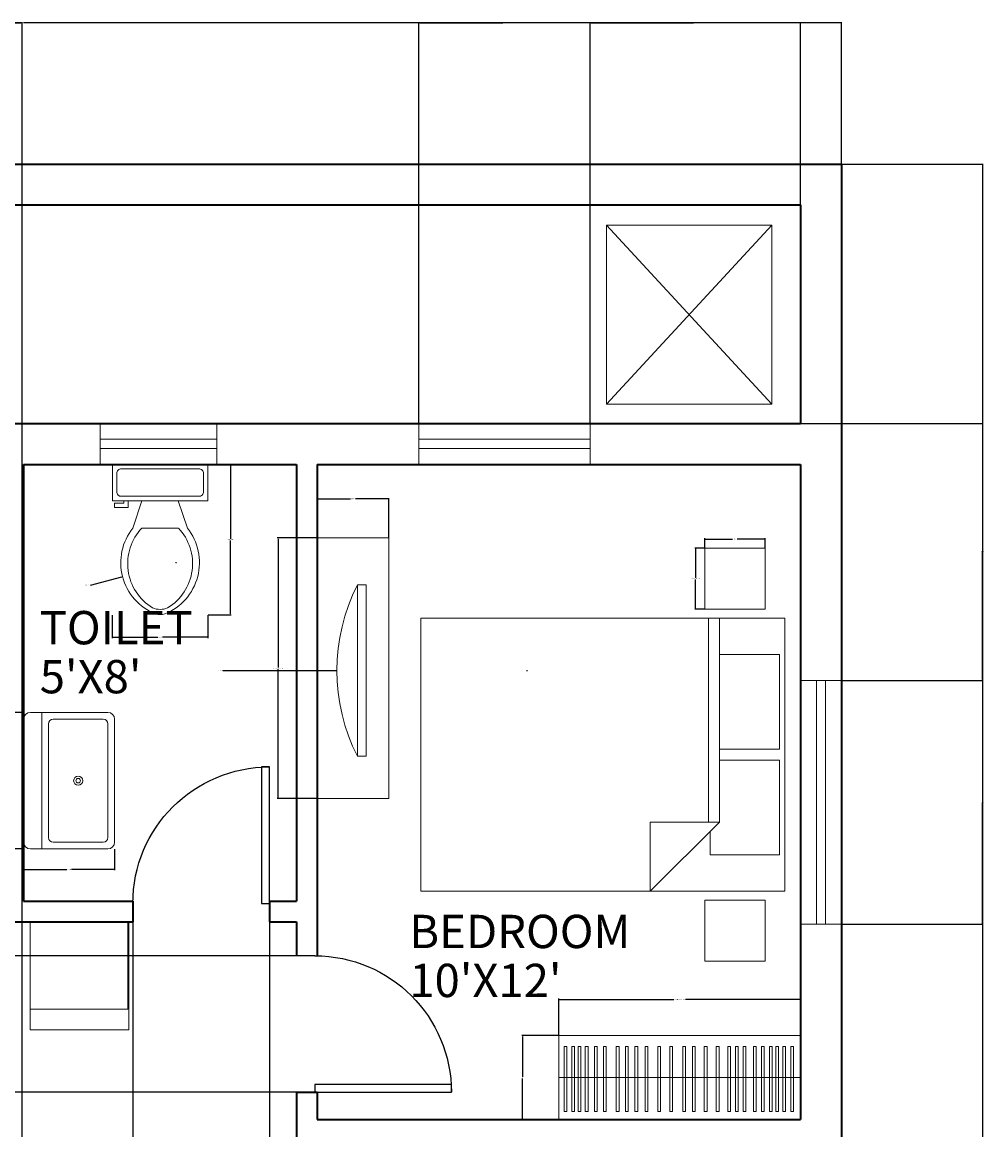
# Model space of a CAD drawing. Units: inches. Extents: x 25018 to 25490, y 41421 to 42101.
# Tile 5 of 5: x 25279 to 25490, y 41858 to 42101. Entities that reach past the tile are written whole.
import ezdxf

# ---------------------------------------------------------------- set-up
doc = ezdxf.new("R2010")
doc.units = ezdxf.units.IN
for name, color, linetype, lineweight in [('A-ANNO-DIMS', 2, 'Continuous', 18), ('A-AREA-IDEN', 7, 'Continuous', 18), ('A-DOOR', 3, 'Continuous', 25), ('A-FLOR-FIXT', 9, 'Continuous', 18), ('A-FURN', 8, 'Continuous', 18), ('A-GLAZ', 4, 'Continuous', 18), ('A-WALL', 7, 'Continuous', 35)]:
    doc.layers.add(name, color=color, linetype=linetype, lineweight=lineweight)
doc.styles.get("Standard").update_dxf_attribs({"font": 'arial.ttf'})
doc.dimstyles.get("Standard").update_dxf_attribs({"dimtxt": 0.18, "dimasz": 0.18, "dimexe": 0.18, "dimexo": 0.0625, "dimgap": 0.09, "dimtad": 0, "dimtih": 1, "dimtoh": 1, "dimdec": 4, "dimzin": 0, "dimdsep": 46, "dimtxsty": 'Standard', "dimcen": 0.09, "dimadec": 0, "dimazin": 0, "dimtfac": 1, "dimtdec": 4, "dimtofl": 0, "dimtmove": 0, "dimatfit": 3, "dimfxl": 1, "dimtolj": 1, "dimtzin": 0, "dimarcsym": 0})

# ---------------------------------------------------------------- blocks, each defined once
blk = doc.blocks.new('*U2')
for p, q in [((0, 0), (0, -100)), ((750, 0), (750, -100))]:
    blk.add_line(p, q)
blk.add_lwpolyline([(0, 0), (0, 750), (43.75, 750), (43.75, 0)], close=True)
blk.add_arc((0, 0), 750, 0, 90)
blk = doc.blocks.new('Toilet - top')
for p, q in [((9.5, -6), (9.5, -2)), ((-10, -8.5), (-8, -8.5)), ((-10, -9.5), (-10, -8.5)), ((-7, -9.5), (-10, -9.5)), ((-8, -8.5), (-8, -8)), ((-7, -8), (-7, -9.5)), ((-4, -8), (-6, -14)), ((4, -8), (6, -14)), ((4, -14), (-4, -14))]:
    blk.add_line(p, q)
blk.add_lwpolyline([(10.5, -8), (10.5, 0), (-10.5, 0), (-10.5, -8)], close=True)
for points in [[(-9.5, -2), (-9.5, -6)], [(8.5, -1), (-8.5, -1)], [(-8.5, -7), (8.5, -7)]]:
    blk.add_lwpolyline(points)
for centre, radius, start, end in [((-8.62, -1.88), 0.884, 81.8699, 188.1301), ((8.62, -1.88), 0.884, 351.8699, 98.1301), ((-8.62, -6.12), 0.884, 171.8699, 278.1301), ((8.62, -6.12), 0.884, 261.8699, 8.1301), ((3.52, -21.58), 12.17, 141.4691, 247.9714), ((4.2, -21.82), 11.33, 136.3677, 238.9468), ((-3.52, -21.58), 12.17, 292.0284, 38.5307), ((-4.2, -21.82), 11.33, 301.053, 43.6321), ((0, -27.88), 4, 245.7318, 294.2682), ((0, -29), 4, 254.8605, 285.1395)]:
    blk.add_arc(centre, radius, start, end)
blk = doc.blocks.new('Sink-single - 30 in top')
blk.add_line((-15, -3.999996), (15, -3.999996))
for points in [[(-13.5, 0), (13.5, 0)], [(-15, -18.499996), (-15, -1.5)], [(15, -1.5), (15, -18.499996)], [(-13.5, -17.499996), (-13.5, -6.499996)], [(-12.5, -5.499996), (12.5, -5.499996)], [(13.5, -6.499996), (13.5, -17.499996)], [(12.5, -18.499996), (-12.5, -18.499996)], [(13.5, -19.999996), (-13.5, -19.999996)]]:
    blk.add_lwpolyline(points)
for radius in [1, 0.5]:
    blk.add_circle((0, -11.999996), radius)
for centre, radius, start, end in [((-13.5, -1.5), 1.5, 90, 180), ((13.5, -1.5), 1.5, 0, 90), ((-12.5, -6.499996), 1, 90, 180), ((12.5, -6.499996), 1, 0, 90), ((-13.5, -18.499996), 1.5, 180, 270), ((-12.5, -17.499996), 1, 180, 270), ((12.5, -17.499996), 1, 270, 0), ((13.5, -18.499996), 1.5, 270, 0)]:
    blk.add_arc(centre, radius, start, end)
blk = doc.blocks.new('Bed - Queen')
for p, q in [((0, -80.00003), (0, 0)), ((0, 0), (59.99999, 0)), ((59.99999, 0), (59.99999, -80.00003)), ((7.99999, -1.2), (28.79998, -1.2)), ((7.99999, -14.4), (7.99999, -1.2)), ((28.79998, -1.2), (28.79998, -14.4)), ((31.19999, -1.2), (51.99999, -1.2)), ((31.19999, -14.4), (31.19999, -1.2)), ((51.99999, -1.2), (51.99999, -16.4)), ((0, -14.4), (44.8, -14.4)), ((59.99999, -29.6), (44.8, -14.4)), ((44.8, -14.4), (44.8, -29.6)), ((44.8, -16.8), (0, -16.8)), ((51.99999, -16.4), (46.79936, -16.4)), ((44.8, -29.6), (59.99999, -29.6)), ((59.99999, -80.00003), (0, -80.00003))]:
    blk.add_line(p, q)
blk = doc.blocks.new('WARDROBE-SLATTED')
blk.add_line((0, 9.22), (53.1, 9.22))
for points in [[(0, 0), (53.1, 0), (53.1, 18.45), (0, 18.45)], [(1.16, 16.06), (1.76, 16.06), (1.76, 1.75), (1.16, 1.75)], [(2.87, 16.06), (3.47, 16.06), (3.47, 1.75), (2.87, 1.75)], [(4.23, 16.06), (4.83, 16.06), (4.83, 1.75), (4.23, 1.75)], [(5.83, 16.06), (6.43, 16.06), (6.43, 1.75), (5.83, 1.75)], [(7.85, 16.06), (8.45, 16.06), (8.45, 1.75), (7.85, 1.75)], [(9.82, 16.06), (10.42, 16.06), (10.42, 1.75), (9.82, 1.75)], [(12.64, 16.06), (13.24, 16.06), (13.24, 1.75), (12.64, 1.75)], [(14.63, 16.06), (15.23, 16.06), (15.23, 1.75), (14.63, 1.75)], [(16.74, 16.06), (17.34, 16.06), (17.34, 1.75), (16.74, 1.75)], [(18.99, 16.06), (19.59, 16.06), (19.59, 1.75), (18.99, 1.75)], [(21.77, 16.06), (22.37, 16.06), (22.37, 1.75), (21.77, 1.75)], [(24.4, 16.06), (25, 16.06), (25, 1.75), (24.4, 1.75)], [(27.25, 16.06), (27.85, 16.06), (27.85, 1.75), (27.25, 1.75)], [(29.36, 16.06), (29.96, 16.06), (29.96, 1.75), (29.36, 1.75)], [(31.98, 16.06), (32.58, 16.06), (32.58, 1.75), (31.98, 1.75)], [(34.61, 16.06), (35.21, 16.06), (35.21, 1.75), (34.61, 1.75)], [(37.17, 16.06), (37.77, 16.06), (37.77, 1.75), (37.17, 1.75)], [(38.82, 16.06), (39.42, 16.06), (39.42, 1.75), (38.82, 1.75)], [(40.51, 16.06), (41.11, 16.06), (41.11, 1.75), (40.51, 1.75)], [(42.78, 16.06), (43.38, 16.06), (43.38, 1.75), (42.78, 1.75)], [(44.55, 16.06), (45.15, 16.06), (45.15, 1.75), (44.55, 1.75)], [(46.32, 16.06), (46.92, 16.06), (46.92, 1.75), (46.32, 1.75)], [(47.7, 16.06), (48.3, 16.06), (48.3, 1.75), (47.7, 1.75)], [(49.2, 16.06), (49.8, 16.06), (49.8, 1.75), (49.2, 1.75)], [(50.97, 16.06), (51.57, 16.06), (51.57, 1.75), (50.97, 1.75)]]:
    blk.add_lwpolyline(points, close=True)
blk = doc.blocks.new('TABLE-BEDSIDE')
blk.add_lwpolyline([(0, 13.4), (13.26, 13.4), (13.26, 0), (0, 0)], close=True)
blk = doc.blocks.new('TV-CONSOLE')
for points in [[(0, 57.27), (15.78, 57.27), (15.78, 0), (0, 0)], [(8.85, 46.95), (10.77, 46.95), (10.77, 9.28), (8.85, 9.28)]]:
    blk.add_lwpolyline(points, close=True)
blk.add_arc((46.16, 28.12), 41.8, 153.2115, 206.7885)
blk = doc.blocks.new('WIN-BATH')
for p, q in [((0, 9), (0, 0)), ((25.67, 0), (25.67, 9)), ((0, 5.5), (25.67, 5.5)), ((0, 3.5), (25.67, 3.5))]:
    blk.add_line(p, q)
blk = doc.blocks.new('*D20')
at = {"layer": 'A-ANNO-DIMS', "color": 0, "lineweight": -2, "transparency": 16777216}
for p, q in [((25396.55, 41878.56), (25396.55, 41886.64)), ((25396.73, 41886.46), (25421.8, 41886.46)), ((25449.47, 41886.46), (25424.41, 41886.46)), ((25449.65, 41878.56), (25449.65, 41886.64))]:
    blk.add_line(p, q, dxfattribs=at)
at = {"layer": 'A-ANNO-DIMS', "color": 0, "transparency": 16777216}
for points in [[(25396.73, 41886.49), (25396.73, 41886.43), (25396.55, 41886.46)], [(25449.47, 41886.49), (25449.47, 41886.43), (25449.65, 41886.46)]]:
    blk.add_solid(points, dxfattribs=at)
at = {"layer": 'Defpoints', "color": 0, "transparency": 16777216}
for p in [(25449.65, 41886.46), (25396.55, 41878.5), (25449.65, 41878.5)]:
    blk.add_point(p, dxfattribs=at)
at = {"layer": 'A-ANNO-DIMS', "color": 0, "transparency": 16777216, "insert": (25423.1, 41886.46), "char_height": 0.18, "attachment_point": 5}
blk.add_mtext('\\A1;WARDROBE 53 TYP.', dxfattribs=at)
blk = doc.blocks.new('*D21')
at = {"layer": 'A-ANNO-DIMS', "color": 0, "lineweight": -2, "transparency": 16777216}
for p, q in [((25396.49, 41878.5), (25388.41, 41878.5)), ((25388.59, 41878.32), (25388.59, 41869.46)), ((25388.59, 41860.23), (25388.59, 41869.09)), ((25396.49, 41860.05), (25388.41, 41860.05))]:
    blk.add_line(p, q, dxfattribs=at)
at = {"layer": 'A-ANNO-DIMS', "color": 0, "transparency": 16777216}
for points in [[(25388.56, 41878.32), (25388.62, 41878.32), (25388.59, 41878.5)], [(25388.56, 41860.23), (25388.62, 41860.23), (25388.59, 41860.05)]]:
    blk.add_solid(points, dxfattribs=at)
at = {"layer": 'Defpoints', "color": 0, "transparency": 16777216}
for p in [(25388.59, 41878.5), (25396.55, 41878.5), (25396.55, 41860.05)]:
    blk.add_point(p, dxfattribs=at)
at = {"layer": 'A-ANNO-DIMS', "color": 0, "transparency": 16777216, "insert": (25388.59, 41869.27), "char_height": 0.18, "attachment_point": 5}
blk.add_mtext('\\A1;18 TYP.', dxfattribs=at)
blk = doc.blocks.new('*D22')
at = {"layer": 'A-ANNO-DIMS', "color": 0, "lineweight": -2, "transparency": 16777216}
for p, q in [((25428.57, 41985.63), (25426.44, 41985.63)), ((25426.62, 41985.45), (25426.62, 41979.12)), ((25426.62, 41972.41), (25426.62, 41978.75)), ((25428.57, 41972.23), (25426.44, 41972.23))]:
    blk.add_line(p, q, dxfattribs=at)
at = {"layer": 'A-ANNO-DIMS', "color": 0, "transparency": 16777216}
for points in [[(25426.59, 41985.45), (25426.65, 41985.45), (25426.62, 41985.63)], [(25426.59, 41972.41), (25426.65, 41972.41), (25426.62, 41972.23)]]:
    blk.add_solid(points, dxfattribs=at)
at = {"layer": 'Defpoints', "color": 0, "transparency": 16777216}
for p in [(25426.62, 41985.63), (25428.63, 41985.63), (25428.63, 41972.23)]:
    blk.add_point(p, dxfattribs=at)
at = {"layer": 'A-ANNO-DIMS', "color": 0, "transparency": 16777216, "insert": (25426.62, 41978.93), "char_height": 0.18, "attachment_point": 5}
blk.add_mtext('\\A1;NIGHTSTAND 13 TYP.', dxfattribs=at)
blk = doc.blocks.new('*D23')
at = {"layer": 'A-ANNO-DIMS', "color": 0, "lineweight": -2, "transparency": 16777216}
for p, q in [((25428.63, 41985.7), (25428.63, 41987.82)), ((25428.81, 41987.64), (25434.74, 41987.64)), ((25441.71, 41987.64), (25435.78, 41987.64)), ((25441.89, 41985.7), (25441.89, 41987.82))]:
    blk.add_line(p, q, dxfattribs=at)
at = {"layer": 'A-ANNO-DIMS', "color": 0, "transparency": 16777216}
for points in [[(25428.81, 41987.67), (25428.81, 41987.61), (25428.63, 41987.64)], [(25441.71, 41987.67), (25441.71, 41987.61), (25441.89, 41987.64)]]:
    blk.add_solid(points, dxfattribs=at)
at = {"layer": 'Defpoints', "color": 0, "transparency": 16777216}
for p in [(25441.89, 41987.64), (25428.63, 41985.63), (25441.89, 41985.63)]:
    blk.add_point(p, dxfattribs=at)
at = {"layer": 'A-ANNO-DIMS', "color": 0, "transparency": 16777216, "insert": (25435.26, 41987.64), "char_height": 0.18, "attachment_point": 5}
blk.add_mtext('\\A1;13 TYP.', dxfattribs=at)
blk = doc.blocks.new('*D24')
at = {"layer": 'A-ANNO-DIMS', "color": 0, "lineweight": -2, "transparency": 16777216}
for p, q in [((25343.39, 41987.88), (25334.68, 41987.88)), ((25334.86, 41987.7), (25334.86, 41959.43)), ((25334.86, 41930.79), (25334.86, 41959.06)), ((25343.39, 41930.61), (25334.68, 41930.61))]:
    blk.add_line(p, q, dxfattribs=at)
at = {"layer": 'A-ANNO-DIMS', "color": 0, "transparency": 16777216}
for points in [[(25334.83, 41987.7), (25334.89, 41987.7), (25334.86, 41987.88)], [(25334.83, 41930.79), (25334.89, 41930.79), (25334.86, 41930.61)]]:
    blk.add_solid(points, dxfattribs=at)
at = {"layer": 'Defpoints', "color": 0, "transparency": 16777216}
for p in [(25334.86, 41987.88), (25343.45, 41987.88), (25343.45, 41930.61)]:
    blk.add_point(p, dxfattribs=at)
at = {"layer": 'A-ANNO-DIMS', "color": 0, "transparency": 16777216, "insert": (25334.86, 41959.24), "char_height": 0.18, "attachment_point": 5}
blk.add_mtext('\\A1;TV CONSOLE 57 TYP.', dxfattribs=at)
blk = doc.blocks.new('*D25')
at = {"layer": 'A-ANNO-DIMS', "color": 0, "lineweight": -2, "transparency": 16777216}
for p, q in [((25343.45, 41987.94), (25343.45, 41996.65)), ((25359.23, 41987.94), (25359.23, 41996.65)), ((25343.63, 41996.47), (25350.82, 41996.47)), ((25359.05, 41996.47), (25351.86, 41996.47))]:
    blk.add_line(p, q, dxfattribs=at)
at = {"layer": 'A-ANNO-DIMS', "color": 0, "transparency": 16777216}
for points in [[(25343.63, 41996.5), (25343.63, 41996.44), (25343.45, 41996.47)], [(25359.05, 41996.5), (25359.05, 41996.44), (25359.23, 41996.47)]]:
    blk.add_solid(points, dxfattribs=at)
at = {"layer": 'Defpoints', "color": 0, "transparency": 16777216}
for p in [(25359.23, 41996.47), (25343.45, 41987.88), (25359.23, 41987.88)]:
    blk.add_point(p, dxfattribs=at)
at = {"layer": 'A-ANNO-DIMS', "color": 0, "transparency": 16777216, "insert": (25351.34, 41996.47), "char_height": 0.18, "attachment_point": 5}
blk.add_mtext('\\A1;16 TYP.', dxfattribs=at)
blk = doc.blocks.new('*D28')
at = {"layer": 'A-ANNO-DIMS', "color": 0, "lineweight": -2, "transparency": 16777216}
for p, q in [((25319.52, 42004.05), (25324.59, 42004.05)), ((25324.41, 42003.87), (25324.41, 41987.71)), ((25324.41, 41971.18), (25324.41, 41987.34)), ((25319.52, 41971), (25324.59, 41971))]:
    blk.add_line(p, q, dxfattribs=at)
at = {"layer": 'A-ANNO-DIMS', "color": 0, "transparency": 16777216}
for points in [[(25324.38, 42003.87), (25324.44, 42003.87), (25324.41, 42004.05)], [(25324.38, 41971.18), (25324.44, 41971.18), (25324.41, 41971)]]:
    blk.add_solid(points, dxfattribs=at)
at = {"layer": 'Defpoints', "color": 0, "transparency": 16777216}
for p in [(25319.45, 42004.05), (25324.41, 42004.05), (25319.45, 41971)]:
    blk.add_point(p, dxfattribs=at)
at = {"layer": 'A-ANNO-DIMS', "color": 0, "transparency": 16777216, "insert": (25324.41, 41987.53), "char_height": 0.18, "attachment_point": 5}
blk.add_mtext('\\A1;WC 33 TYP.', dxfattribs=at)
blk = doc.blocks.new('*D29')
at = {"layer": 'A-ANNO-DIMS', "color": 0, "lineweight": -2, "transparency": 16777216}
for p, q in [((25298.45, 41970.94), (25298.45, 41965.87)), ((25319.45, 41970.94), (25319.45, 41965.87)), ((25298.63, 41966.05), (25308.42, 41966.05)), ((25319.27, 41966.05), (25309.48, 41966.05))]:
    blk.add_line(p, q, dxfattribs=at)
at = {"layer": 'A-ANNO-DIMS', "color": 0, "transparency": 16777216}
for points in [[(25298.63, 41966.08), (25298.63, 41966.02), (25298.45, 41966.05)], [(25319.27, 41966.08), (25319.27, 41966.02), (25319.45, 41966.05)]]:
    blk.add_solid(points, dxfattribs=at)
at = {"layer": 'Defpoints', "color": 0, "transparency": 16777216}
for p in [(25298.45, 41971), (25319.45, 41971), (25319.45, 41966.05)]:
    blk.add_point(p, dxfattribs=at)
at = {"layer": 'A-ANNO-DIMS', "color": 0, "transparency": 16777216, "insert": (25308.95, 41966.05), "char_height": 0.18, "attachment_point": 5}
blk.add_mtext('\\A1;21 TYP.', dxfattribs=at)
blk = doc.blocks.new('*D30')
at = {"layer": 'A-ANNO-DIMS', "color": 0, "lineweight": -2, "transparency": 16777216}
for p, q in [((25278.89, 41949.53), (25274.27, 41949.53)), ((25274.45, 41949.35), (25274.45, 41934.71)), ((25274.45, 41919.71), (25274.45, 41934.35)), ((25278.89, 41919.53), (25274.27, 41919.53))]:
    blk.add_line(p, q, dxfattribs=at)
at = {"layer": 'A-ANNO-DIMS', "color": 0, "transparency": 16777216}
for points in [[(25274.42, 41949.35), (25274.48, 41949.35), (25274.45, 41949.53)], [(25274.42, 41919.71), (25274.48, 41919.71), (25274.45, 41919.53)]]:
    blk.add_solid(points, dxfattribs=at)
at = {"layer": 'Defpoints', "color": 0, "transparency": 16777216}
for p in [(25274.45, 41949.53), (25278.95, 41949.53), (25278.95, 41919.53)]:
    blk.add_point(p, dxfattribs=at)
at = {"layer": 'A-ANNO-DIMS', "color": 0, "transparency": 16777216, "insert": (25274.45, 41934.53), "char_height": 0.18, "attachment_point": 5}
blk.add_mtext('\\A1;BASIN 30 TYP.', dxfattribs=at)
blk = doc.blocks.new('*D31')
at = {"layer": 'A-ANNO-DIMS', "color": 0, "lineweight": -2, "transparency": 16777216}
for p, q in [((25278.95, 41919.47), (25278.95, 41914.85)), ((25298.95, 41919.47), (25298.95, 41914.85)), ((25279.13, 41915.03), (25288.42, 41915.03)), ((25298.77, 41915.03), (25289.48, 41915.03))]:
    blk.add_line(p, q, dxfattribs=at)
at = {"layer": 'A-ANNO-DIMS', "color": 0, "transparency": 16777216}
for points in [[(25279.13, 41915.06), (25279.13, 41915), (25278.95, 41915.03)], [(25298.77, 41915.06), (25298.77, 41915), (25298.95, 41915.03)]]:
    blk.add_solid(points, dxfattribs=at)
at = {"layer": 'Defpoints', "color": 0, "transparency": 16777216}
for p in [(25278.95, 41919.53), (25298.95, 41919.53), (25278.95, 41915.03)]:
    blk.add_point(p, dxfattribs=at)
at = {"layer": 'A-ANNO-DIMS', "color": 0, "transparency": 16777216, "insert": (25288.95, 41915.03), "char_height": 0.18, "attachment_point": 5}
blk.add_mtext('\\A1;20 TYP.', dxfattribs=at)
blk = doc.blocks.new('*D38')
at = {"layer": 'A-ANNO-DIMS', "color": 0, "lineweight": -2, "transparency": 16777216}
for p, q in [((25098.65, 42070.11), (25098.65, 42101.23)), ((25458.65, 42070.11), (25458.65, 42101.23)), ((25098.83, 42101.05), (25278.36, 42101.05)), ((25458.47, 42101.05), (25278.94, 42101.05))]:
    blk.add_line(p, q, dxfattribs=at)
at = {"layer": 'A-ANNO-DIMS', "color": 0, "transparency": 16777216}
for points in [[(25098.83, 42101.08), (25098.83, 42101.02), (25098.65, 42101.05)], [(25458.47, 42101.08), (25458.47, 42101.02), (25458.65, 42101.05)]]:
    blk.add_solid(points, dxfattribs=at)
at = {"layer": 'Defpoints', "color": 0, "transparency": 16777216}
for p in [(25458.65, 42101.05), (25098.65, 42070.05), (25458.65, 42070.05)]:
    blk.add_point(p, dxfattribs=at)
at = {"layer": 'A-ANNO-DIMS', "color": 0, "transparency": 16777216, "insert": (25278.65, 42101.05), "char_height": 0.18, "attachment_point": 5}
blk.add_mtext('\\A1;360', dxfattribs=at)
blk = doc.blocks.new('*D39')
at = {"layer": 'A-ANNO-DIMS', "color": 0, "lineweight": -2, "transparency": 16777216}
for p, q in [((25458.72, 42070.05), (25489.83, 42070.05)), ((25489.65, 42069.87), (25489.65, 41785.98)), ((25489.65, 41501.73), (25489.65, 41785.62)), ((25458.72, 41501.55), (25489.83, 41501.55))]:
    blk.add_line(p, q, dxfattribs=at)
at = {"layer": 'A-ANNO-DIMS', "color": 0, "transparency": 16777216}
for points in [[(25489.62, 42069.87), (25489.68, 42069.87), (25489.65, 42070.05)], [(25489.62, 41501.73), (25489.68, 41501.73), (25489.65, 41501.55)]]:
    blk.add_solid(points, dxfattribs=at)
at = {"layer": 'Defpoints', "color": 0, "transparency": 16777216}
for p in [(25458.65, 42070.05), (25489.65, 42070.05), (25458.65, 41501.55)]:
    blk.add_point(p, dxfattribs=at)
at = {"layer": 'A-ANNO-DIMS', "color": 0, "transparency": 16777216, "insert": (25489.65, 41785.8), "char_height": 0.18, "attachment_point": 5}
blk.add_mtext('\\A1;568.5', dxfattribs=at)
blk = doc.blocks.new('*D56')
at = {"layer": 'A-ANNO-DIMS', "color": 0, "lineweight": -2, "transparency": 16777216}
for p, q in [((25458.72, 41903), (25489.83, 41903)), ((25489.65, 41902.82), (25489.65, 41855.5)), ((25489.65, 41807.81), (25489.65, 41855.13)), ((25458.72, 41807.63), (25489.83, 41807.63))]:
    blk.add_line(p, q, dxfattribs=at)
at = {"layer": 'A-ANNO-DIMS', "color": 0, "transparency": 16777216}
for points in [[(25489.62, 41902.82), (25489.68, 41902.82), (25489.65, 41903)], [(25489.62, 41807.81), (25489.68, 41807.81), (25489.65, 41807.63)]]:
    blk.add_solid(points, dxfattribs=at)
at = {"layer": 'Defpoints', "color": 0, "transparency": 16777216}
for p in [(25458.65, 41903), (25489.65, 41903), (25458.65, 41807.63)]:
    blk.add_point(p, dxfattribs=at)
at = {"layer": 'A-ANNO-DIMS', "color": 0, "transparency": 16777216, "insert": (25489.65, 41855.31), "char_height": 0.18, "attachment_point": 5}
blk.add_mtext('\\A1;95.36', dxfattribs=at)
blk = doc.blocks.new('*D57')
at = {"layer": 'A-ANNO-DIMS', "color": 0, "lineweight": -2, "transparency": 16777216}
for p, q in [((25458.72, 41956.57), (25489.83, 41956.57)), ((25489.65, 41956.39), (25489.65, 41929.96)), ((25489.65, 41903.18), (25489.65, 41929.6)), ((25458.72, 41903), (25489.83, 41903))]:
    blk.add_line(p, q, dxfattribs=at)
at = {"layer": 'A-ANNO-DIMS', "color": 0, "transparency": 16777216}
for points in [[(25489.62, 41956.39), (25489.68, 41956.39), (25489.65, 41956.57)], [(25489.62, 41903.18), (25489.68, 41903.18), (25489.65, 41903)]]:
    blk.add_solid(points, dxfattribs=at)
at = {"layer": 'Defpoints', "color": 0, "transparency": 16777216}
for p in [(25458.65, 41956.57), (25489.65, 41956.57), (25458.65, 41903)]:
    blk.add_point(p, dxfattribs=at)
at = {"layer": 'A-ANNO-DIMS', "color": 0, "transparency": 16777216, "insert": (25489.65, 41929.78), "char_height": 0.18, "attachment_point": 5}
blk.add_mtext('\\A1;53.57', dxfattribs=at)
blk = doc.blocks.new('*D58')
at = {"layer": 'A-ANNO-DIMS', "color": 0, "lineweight": -2, "transparency": 16777216}
for p, q in [((25449.72, 42013.05), (25489.83, 42013.05)), ((25489.65, 42012.87), (25489.65, 41984.99)), ((25489.65, 41956.75), (25489.65, 41984.63)), ((25458.72, 41956.57), (25489.83, 41956.57))]:
    blk.add_line(p, q, dxfattribs=at)
at = {"layer": 'A-ANNO-DIMS', "color": 0, "transparency": 16777216}
for points in [[(25489.62, 42012.87), (25489.68, 42012.87), (25489.65, 42013.05)], [(25489.62, 41956.75), (25489.68, 41956.75), (25489.65, 41956.57)]]:
    blk.add_solid(points, dxfattribs=at)
at = {"layer": 'Defpoints', "color": 0, "transparency": 16777216}
for p in [(25449.65, 42013.05), (25489.65, 42013.05), (25458.65, 41956.57)]:
    blk.add_point(p, dxfattribs=at)
at = {"layer": 'A-ANNO-DIMS', "color": 0, "transparency": 16777216, "insert": (25489.65, 41984.81), "char_height": 0.18, "attachment_point": 5}
blk.add_mtext('\\A1;56.48', dxfattribs=at)
blk = doc.blocks.new('*D64')
at = {"layer": 'A-ANNO-DIMS', "color": 0, "lineweight": -2, "transparency": 16777216}
for p, q in [((25365.82, 42013.11), (25365.82, 42101.23)), ((25403.48, 42013.11), (25403.48, 42101.23)), ((25366, 42101.05), (25384.26, 42101.05)), ((25403.3, 42101.05), (25385.05, 42101.05))]:
    blk.add_line(p, q, dxfattribs=at)
at = {"layer": 'A-ANNO-DIMS', "color": 0, "transparency": 16777216}
for points in [[(25366, 42101.08), (25366, 42101.02), (25365.82, 42101.05)], [(25403.3, 42101.08), (25403.3, 42101.02), (25403.48, 42101.05)]]:
    blk.add_solid(points, dxfattribs=at)
at = {"layer": 'Defpoints', "color": 0, "transparency": 16777216}
for p in [(25403.48, 42101.05), (25365.82, 42013.05), (25403.48, 42013.05)]:
    blk.add_point(p, dxfattribs=at)
at = {"layer": 'A-ANNO-DIMS', "color": 0, "transparency": 16777216, "insert": (25384.65, 42101.05), "char_height": 0.18, "attachment_point": 5}
blk.add_mtext('\\A1;37.66', dxfattribs=at)
blk = doc.blocks.new('*D65')
at = {"layer": 'A-ANNO-DIMS', "color": 0, "lineweight": -2, "transparency": 16777216}
for p, q in [((25403.48, 42013.11), (25403.48, 42101.23)), ((25449.65, 42013.11), (25449.65, 42101.23)), ((25403.66, 42101.05), (25426.17, 42101.05)), ((25449.47, 42101.05), (25426.97, 42101.05))]:
    blk.add_line(p, q, dxfattribs=at)
at = {"layer": 'A-ANNO-DIMS', "color": 0, "transparency": 16777216}
for points in [[(25403.66, 42101.08), (25403.66, 42101.02), (25403.48, 42101.05)], [(25449.47, 42101.08), (25449.47, 42101.02), (25449.65, 42101.05)]]:
    blk.add_solid(points, dxfattribs=at)
at = {"layer": 'Defpoints', "color": 0, "transparency": 16777216}
for p in [(25449.65, 42101.05), (25403.48, 42013.05), (25449.65, 42013.05)]:
    blk.add_point(p, dxfattribs=at)
at = {"layer": 'A-ANNO-DIMS', "color": 0, "transparency": 16777216, "insert": (25426.57, 42101.05), "char_height": 0.18, "attachment_point": 5}
blk.add_mtext('\\A1;46.17', dxfattribs=at)
blk = doc.blocks.new('*D70')
at = {"layer": 'A-ANNO-DIMS', "color": 0, "lineweight": -2, "transparency": 16777216}
for p, q in [((25250.45, 41903.49), (25250.45, 41420.7)), ((25302.95, 41903.49), (25302.95, 41420.7)), ((25250.63, 41420.88), (25276.38, 41420.88)), ((25302.77, 41420.88), (25277.03, 41420.88))]:
    blk.add_line(p, q, dxfattribs=at)
at = {"layer": 'A-ANNO-DIMS', "color": 0, "transparency": 16777216}
for points in [[(25250.63, 41420.91), (25250.63, 41420.85), (25250.45, 41420.88)], [(25302.77, 41420.91), (25302.77, 41420.85), (25302.95, 41420.88)]]:
    blk.add_solid(points, dxfattribs=at)
at = {"layer": 'Defpoints', "color": 0, "transparency": 16777216}
for p in [(25250.45, 41903.55), (25302.95, 41903.55), (25302.95, 41420.88)]:
    blk.add_point(p, dxfattribs=at)
at = {"layer": 'A-ANNO-DIMS', "color": 0, "transparency": 16777216, "insert": (25276.7, 41420.88), "char_height": 0.18, "attachment_point": 5}
blk.add_mtext('\\A1;52.5', dxfattribs=at)
blk = doc.blocks.new('*D71')
at = {"layer": 'A-ANNO-DIMS', "color": 0, "lineweight": -2, "transparency": 16777216}
for p, q in [((25302.95, 41903.49), (25302.95, 41420.7)), ((25332.95, 41903.49), (25332.95, 41420.7)), ((25303.13, 41420.88), (25317.73, 41420.88)), ((25332.77, 41420.88), (25318.17, 41420.88))]:
    blk.add_line(p, q, dxfattribs=at)
at = {"layer": 'A-ANNO-DIMS', "color": 0, "transparency": 16777216}
for points in [[(25303.13, 41420.91), (25303.13, 41420.85), (25302.95, 41420.88)], [(25332.77, 41420.91), (25332.77, 41420.85), (25332.95, 41420.88)]]:
    blk.add_solid(points, dxfattribs=at)
at = {"layer": 'Defpoints', "color": 0, "transparency": 16777216}
for p in [(25302.95, 41903.55), (25332.95, 41903.55), (25332.95, 41420.88)]:
    blk.add_point(p, dxfattribs=at)
at = {"layer": 'A-ANNO-DIMS', "color": 0, "transparency": 16777216, "insert": (25317.95, 41420.88), "char_height": 0.18, "attachment_point": 5}
blk.add_mtext('\\A1;30', dxfattribs=at)
blk = doc.blocks.new('*D72')
at = {"layer": 'A-ANNO-DIMS', "color": 0, "lineweight": -2, "transparency": 16777216}
for p, q in [((25338.89, 41896.05), (25018.58, 41896.05)), ((25018.76, 41895.87), (25018.76, 41881.23)), ((25018.76, 41866.23), (25018.76, 41880.87)), ((25338.89, 41866.05), (25018.58, 41866.05))]:
    blk.add_line(p, q, dxfattribs=at)
at = {"layer": 'A-ANNO-DIMS', "color": 0, "transparency": 16777216}
for points in [[(25018.73, 41895.87), (25018.79, 41895.87), (25018.76, 41896.05)], [(25018.73, 41866.23), (25018.79, 41866.23), (25018.76, 41866.05)]]:
    blk.add_solid(points, dxfattribs=at)
at = {"layer": 'Defpoints', "color": 0, "transparency": 16777216}
for p in [(25018.76, 41896.05), (25338.95, 41896.05), (25338.95, 41866.05)]:
    blk.add_point(p, dxfattribs=at)
at = {"layer": 'A-ANNO-DIMS', "color": 0, "transparency": 16777216, "insert": (25018.76, 41881.05), "char_height": 0.18, "attachment_point": 5}
blk.add_mtext('\\A1;30', dxfattribs=at)
blk = doc.blocks.new('*D75')
at = {"layer": 'A-ANNO-DIMS', "color": 0, "lineweight": -2, "transparency": 16777216}
for p, q in [((25201.64, 41804.94), (25201.64, 42101.23)), ((25278.63, 41804.94), (25278.63, 42101.23)), ((25201.82, 42101.05), (25239.92, 42101.05)), ((25278.45, 42101.05), (25240.36, 42101.05))]:
    blk.add_line(p, q, dxfattribs=at)
at = {"layer": 'A-ANNO-DIMS', "color": 0, "transparency": 16777216}
for points in [[(25201.82, 42101.08), (25201.82, 42101.02), (25201.64, 42101.05)], [(25278.45, 42101.08), (25278.45, 42101.02), (25278.63, 42101.05)]]:
    blk.add_solid(points, dxfattribs=at)
at = {"layer": 'Defpoints', "color": 0, "transparency": 16777216}
for p in [(25278.63, 42101.05), (25201.64, 41804.88), (25278.63, 41804.88)]:
    blk.add_point(p, dxfattribs=at)
at = {"layer": 'A-ANNO-DIMS', "color": 0, "transparency": 16777216, "insert": (25240.14, 42101.05), "char_height": 0.18, "attachment_point": 5}
blk.add_mtext('\\A1;77', dxfattribs=at)
blk = doc.blocks.new('*D77')
at = {"layer": 'A-ANNO-DIMS', "color": 0, "lineweight": -2, "transparency": 16777216}
for p, q in [((25322.74, 41958.72), (25347.64, 41958.72)), ((25389.52, 41958.72), (25389.7, 41958.72)), ((25389.61, 41958.63), (25389.61, 41958.81))]:
    blk.add_line(p, q, dxfattribs=at)
at = {"layer": 'A-ANNO-DIMS', "color": 0, "transparency": 16777216}
blk.add_solid([(25347.64, 41958.75), (25347.64, 41958.69), (25347.82, 41958.72)], dxfattribs=at)
at = {"layer": 'Defpoints', "color": 0, "transparency": 16777216}
for p in [(25347.82, 41958.72), (25389.61, 41958.72)]:
    blk.add_point(p, dxfattribs=at)
at = {"layer": 'A-ANNO-DIMS', "color": 0, "transparency": 16777216, "insert": (25322.13, 41958.72), "char_height": 0.18, "attachment_point": 5}
blk.add_mtext('\\A1;2X R41.8', dxfattribs=at)
blk = doc.blocks.new('*D78')
at = {"layer": 'A-ANNO-DIMS', "color": 0, "lineweight": -2, "transparency": 16777216}
for p, q in [((25312.38, 41982.47), (25312.56, 41982.47)), ((25312.47, 41982.38), (25312.47, 41982.56)), ((25293.64, 41977.52), (25300.53, 41979.33))]:
    blk.add_line(p, q, dxfattribs=at)
at = {"layer": 'A-ANNO-DIMS', "color": 0, "transparency": 16777216}
blk.add_solid([(25300.52, 41979.36), (25300.54, 41979.3), (25300.7, 41979.38)], dxfattribs=at)
at = {"layer": 'Defpoints', "color": 0, "transparency": 16777216}
for p in [(25312.47, 41982.47), (25300.7, 41979.38)]:
    blk.add_point(p, dxfattribs=at)
at = {"layer": 'A-ANNO-DIMS', "color": 0, "transparency": 16777216, "insert": (25292.96, 41977.52), "char_height": 0.18, "attachment_point": 5}
blk.add_mtext('\\A1;4X R12.17', dxfattribs=at)

msp = doc.modelspace()

# ---------------------------------------------------------------- linework, layer by layer
at = {"layer": 'A-FLOR-FIXT'}
for p, q in [((25407.0062, 42017.306), (25443.3638, 42056.6421)), ((25407.0062, 42056.6421), (25443.3638, 42017.306))]:
    msp.add_line(p, q, dxfattribs=at)
for points in [[(25407.0062, 42056.6421), (25443.3638, 42056.6421), (25443.3638, 42017.306), (25407.0062, 42017.306)], [(25280.4079, 41903.5498), (25301.8795, 41903.5498), (25301.8795, 41884.3127), (25280.4079, 41884.3127)], [(25280.4079, 41903.5498), (25302.0898, 41903.5498), (25302.0898, 41879.7836), (25280.4079, 41879.7836)]]:
    msp.add_lwpolyline(points, close=True, dxfattribs=at)
at = {"layer": 'A-GLAZ'}
for p, q in [((25365.8241, 42004.0498), (25365.8241, 42013.0498)), ((25403.483, 42004.0498), (25403.483, 42013.0498)), ((25365.8241, 42009.5498), (25403.483, 42009.5498)), ((25365.8241, 42007.5498), (25403.483, 42007.5498)), ((25449.6526, 41956.5665), (25458.6526, 41956.5665)), ((25453.1526, 41956.5665), (25453.1526, 41902.9968)), ((25455.1526, 41956.5665), (25455.1526, 41902.9968)), ((25449.6526, 41902.9968), (25458.6526, 41902.9968))]:
    msp.add_line(p, q, dxfattribs=at)
at = {"layer": 'A-WALL'}
for p, q in [((25098.6526, 42070.0498), (25458.6526, 42070.0498)), ((25458.6526, 42070.0498), (25458.6526, 41501.5498)), ((25107.6526, 42061.0498), (25449.6526, 42061.0498)), ((25449.6526, 42061.0498), (25449.6526, 42013.0498)), ((25115.4026, 42013.0498), (25449.6526, 42013.0498)), ((25278.9527, 42004.0498), (25278.9527, 41908.0498)), ((25278.9527, 42004.0498), (25338.9527, 42004.0498)), ((25338.9527, 42004.0498), (25338.9527, 41908.0498)), ((25343.4527, 42004.0498), (25343.4527, 41896.0457)), ((25343.4527, 42004.0498), (25449.6526, 42004.0498)), ((25449.6526, 42004.0498), (25449.6526, 41860.0498)), ((25278.9527, 41908.0498), (25302.9527, 41908.0498)), ((25302.9527, 41908.0498), (25302.9527, 41903.5498)), ((25332.9527, 41908.0498), (25332.9527, 41903.5498)), ((25332.9527, 41908.0498), (25338.9527, 41908.0498)), ((25250.4527, 41903.5498), (25302.9527, 41903.5498)), ((25332.9527, 41903.5498), (25338.9527, 41903.5498)), ((25338.9527, 41903.5498), (25338.9527, 41896.0498)), ((25338.9527, 41866.0498), (25343.4527, 41866.0498)), ((25338.9527, 41866.0498), (25338.9527, 41860.0498)), ((25343.4527, 41866.0498), (25343.4527, 41860.0498)), ((25338.9527, 41860.0498), (25338.9527, 41855.5498)), ((25343.4527, 41860.0498), (25449.6526, 41860.0498))]:
    msp.add_line(p, q, dxfattribs=at)

# ---------------------------------------------------------------- block references
at = {"layer": 'A-DOOR', "xscale": -0.0400000000000011, "yscale": 0.0400000000000011, "zscale": 0.0400000000000011}
msp.add_blockref('*U2', (25332.9527, 41907.5498), dxfattribs=at)
at = {"layer": 'A-DOOR', "xscale": -0.0400000000000011, "yscale": 0.0400000000000011, "zscale": 0.0400000000000011, "rotation": 270}
msp.add_blockref('*U2', (25342.9527, 41866.0498), dxfattribs=at)
at = {"layer": 'A-FLOR-FIXT'}
msp.add_blockref('Toilet - top', (25308.9527, 42004.0498), dxfattribs=at)
at = {"layer": 'A-FLOR-FIXT', "rotation": 90}
msp.add_blockref('Sink-single - 30 in top', (25278.9527, 41934.5291), dxfattribs=at)
at = {"layer": 'A-FURN'}
for name, p in [('TV-CONSOLE', (25343.4531, 41930.6073)), ('TABLE-BEDSIDE', (25428.629, 41972.231)), ('WARDROBE-SLATTED', (25396.553, 41860.05))]:
    msp.add_blockref(name, p, dxfattribs=at)
at = {"layer": 'A-FURN', "rotation": 270}
msp.add_blockref('Bed - Queen', (25446.2521, 41970.2529), dxfattribs=at)
at = {"layer": 'A-FURN', "extrusion": (0, 0, -1), "zscale": -1, "rotation": 180}
msp.add_blockref('TABLE-BEDSIDE', (-25428.629, 41908.2748), dxfattribs=at)
at = {"layer": 'A-GLAZ'}
msp.add_blockref('WIN-BATH', (25295.751, 42004.05), dxfattribs=at)

# ---------------------------------------------------------------- texts
at = {"layer": 'A-AREA-IDEN'}
for s, p in [('TOILET', (25282.4936, 41964.4979)), ("5'X8'", (25282.5012, 41953.7386)), ('BEDROOM', (25363.7074, 41897.7354)), ("10'X12'", (25363.715, 41886.9762))]:
    msp.add_text(s, height=7.32047, dxfattribs=at).set_placement(p)

# ---------------------------------------------------------------- dimensions: what is measured, and where the dimension line sits
at = {"layer": 'A-ANNO-DIMS'}
for base, p1, p2, override, picture, middle in [((25458.6526, 42101.0498), (25098.6526, 42070.0498), (25458.6526, 42070.0498), {"dimdec": 0, "dimlfac": 1, "dimrnd": 0, "dimzin": 0, "dimdsep": 46, "dimlunit": 2}, '*D38', (25278.6526, 42101.0498)), ((25278.6341, 42101.0498), (25201.6418, 41804.8791), (25278.6341, 41804.8791), {"dimdec": 0, "dimlfac": 1, "dimrnd": 0, "dimzin": 0, "dimdsep": 46, "dimlunit": 2}, '*D75', (25240.138, 42101.0498)), ((25403.483, 42101.0498), (25365.8241, 42013.0498), (25403.483, 42013.0498), {"dimdec": 2, "dimlfac": 1, "dimrnd": 0, "dimzin": 0, "dimdsep": 46, "dimlunit": 2}, '*D64', (25384.6536, 42101.0498)), ((25449.6526, 42101.0498), (25403.483, 42013.0498), (25449.6526, 42013.0498), {"dimdec": 2, "dimlfac": 1, "dimrnd": 0, "dimzin": 0, "dimdsep": 46, "dimlunit": 2}, '*D65', (25426.5678, 42101.0498)), ((25302.9527, 41420.8835), (25250.4527, 41903.5498), (25302.9527, 41903.5498), {"dimdec": 1, "dimlfac": 1, "dimrnd": 0, "dimzin": 0, "dimdsep": 46, "dimlunit": 2}, '*D70', (25276.7027, 41420.8835)), ((25332.9527, 41420.8835), (25302.9527, 41903.5498), (25332.9527, 41903.5498), {"dimdec": 0, "dimlfac": 1, "dimrnd": 0, "dimzin": 0, "dimdsep": 46, "dimlunit": 2}, '*D71', (25317.9527, 41420.8835))]:
    dim = msp.add_linear_dim(base=base, p1=p1, p2=p2, dimstyle='Standard', override=override, dxfattribs=at)
    dim.commit()
    dim.dimension.update_dxf_attribs({"geometry": picture, "text_midpoint": middle})
for base, p1, p2, override, picture, middle in [((25489.6526, 42070.0498), (25458.6526, 41501.5498), (25458.6526, 42070.0498), {"dimdec": 1, "dimlfac": 1, "dimrnd": 0, "dimzin": 0, "dimdsep": 46, "dimlunit": 2}, '*D39', (25489.6526, 41785.7998)), ((25489.6526, 42013.0498), (25458.6526, 41956.5665), (25449.6526, 42013.0498), {"dimdec": 2, "dimlfac": 1, "dimrnd": 0, "dimzin": 0, "dimdsep": 46, "dimlunit": 2}, '*D58', (25489.6526, 41984.8081)), ((25489.6526, 41956.5665), (25458.6526, 41902.9968), (25458.6526, 41956.5665), {"dimdec": 2, "dimlfac": 1, "dimrnd": 0, "dimzin": 0, "dimdsep": 46, "dimlunit": 2}, '*D57', (25489.6526, 41929.7816)), ((25489.6526, 41902.9968), (25458.6526, 41807.6331), (25458.6526, 41902.9968), {"dimdec": 2, "dimlfac": 1, "dimrnd": 0, "dimzin": 0, "dimdsep": 46, "dimlunit": 2}, '*D56', (25489.6526, 41855.315)), ((25018.7568, 41896.0498), (25338.9527, 41866.0498), (25338.9527, 41896.0498), {"dimdec": 0, "dimlfac": 1, "dimrnd": 0, "dimzin": 0, "dimdsep": 46, "dimlunit": 2}, '*D72', (25018.7568, 41881.0498))]:
    dim = msp.add_linear_dim(base=base, p1=p1, p2=p2, angle=90, dimstyle='Standard', override=override, dxfattribs=at)
    dim.commit()
    dim.dimension.update_dxf_attribs({"geometry": picture, "text_midpoint": middle})
for base, p1, p2, angle, text, picture, middle in [((25324.4096, 42004.0498), (25319.4527, 41971.0036), (25319.4527, 42004.0498), 90, 'WC <> TYP.', '*D28', (25324.4096, 41987.5267)), ((25334.8619, 41987.8788), (25343.4527, 41930.607), (25343.4527, 41987.8788), 90, 'TV CONSOLE <> TYP.', '*D24', (25334.8619, 41959.2429)), ((25426.6188, 41985.6335), (25428.6291, 41972.2314), (25428.6291, 41985.6335), 90, 'NIGHTSTAND <> TYP.', '*D22', (25426.6188, 41978.9325)), ((25274.4527, 41949.5291), (25278.9527, 41919.5291), (25278.9527, 41949.5291), 90, 'BASIN <> TYP.', '*D30', (25274.4527, 41934.5291)), ((25278.9527, 41915.0291), (25298.9527, 41919.5291), (25278.9527, 41919.5291), 180, '<> TYP.', '*D31', (25288.9527, 41915.0291)), ((25388.5877, 41878.4971), (25396.5527, 41860.0498), (25396.5527, 41878.4971), 90, '<> TYP.', '*D21', (25388.5877, 41869.2735))]:
    dim = msp.add_linear_dim(base=base, p1=p1, p2=p2, angle=angle, text=text, dimstyle='Standard', override={"dimdec": 0, "dimlfac": 1, "dimrnd": 0, "dimzin": 0, "dimdsep": 46, "dimlunit": 2}, dxfattribs=at)
    dim.commit()
    dim.dimension.update_dxf_attribs({"geometry": picture, "text_midpoint": middle})
for base, p1, p2, text, picture, middle in [((25359.2332, 41996.4696), (25343.4527, 41987.8788), (25359.2332, 41987.8788), '<> TYP.', '*D25', (25351.343, 41996.4696)), ((25441.8908, 41987.6438), (25428.6291, 41985.6335), (25441.8908, 41985.6335), '<> TYP.', '*D23', (25435.2599, 41987.6438)), ((25319.4527, 41966.0467), (25298.4527, 41971.0036), (25319.4527, 41971.0036), '<> TYP.', '*D29', (25308.9527, 41966.0467)), ((25449.6526, 41886.4621), (25396.5527, 41878.4971), (25449.6526, 41878.4971), 'WARDROBE <> TYP.', '*D20', (25423.1026, 41886.4621))]:
    dim = msp.add_linear_dim(base=base, p1=p1, p2=p2, text=text, dimstyle='Standard', override={"dimdec": 0, "dimlfac": 1, "dimrnd": 0, "dimzin": 0, "dimdsep": 46, "dimlunit": 2}, dxfattribs=at)
    dim.commit()
    dim.dimension.update_dxf_attribs({"geometry": picture, "text_midpoint": middle})
for center, mpoint, text, override, picture, middle in [((25312.4723, 41982.4693), (25300.7027, 41979.3769), '4X <>', {"dimdec": 2, "dimlfac": 1, "dimrnd": 0, "dimzin": 0, "dimdsep": 46, "dimlunit": 2}, '*D78', (25293.641, 41977.5215)), ((25389.6121, 41958.7245), (25347.8158, 41958.724), '2X <>', {"dimdec": 1, "dimlfac": 1, "dimrnd": 0, "dimzin": 0, "dimdsep": 46, "dimlunit": 2}, '*D77', (25322.738, 41958.7237))]:
    dim = msp.add_radius_dim(center=center, mpoint=mpoint, text=text, dimstyle='Standard', override=override, dxfattribs=at)
    dim.commit()
    dim.dimension.update_dxf_attribs({"geometry": picture, "text_midpoint": middle, "dimtype": 164})

doc.saveas('drawing.dxf')
